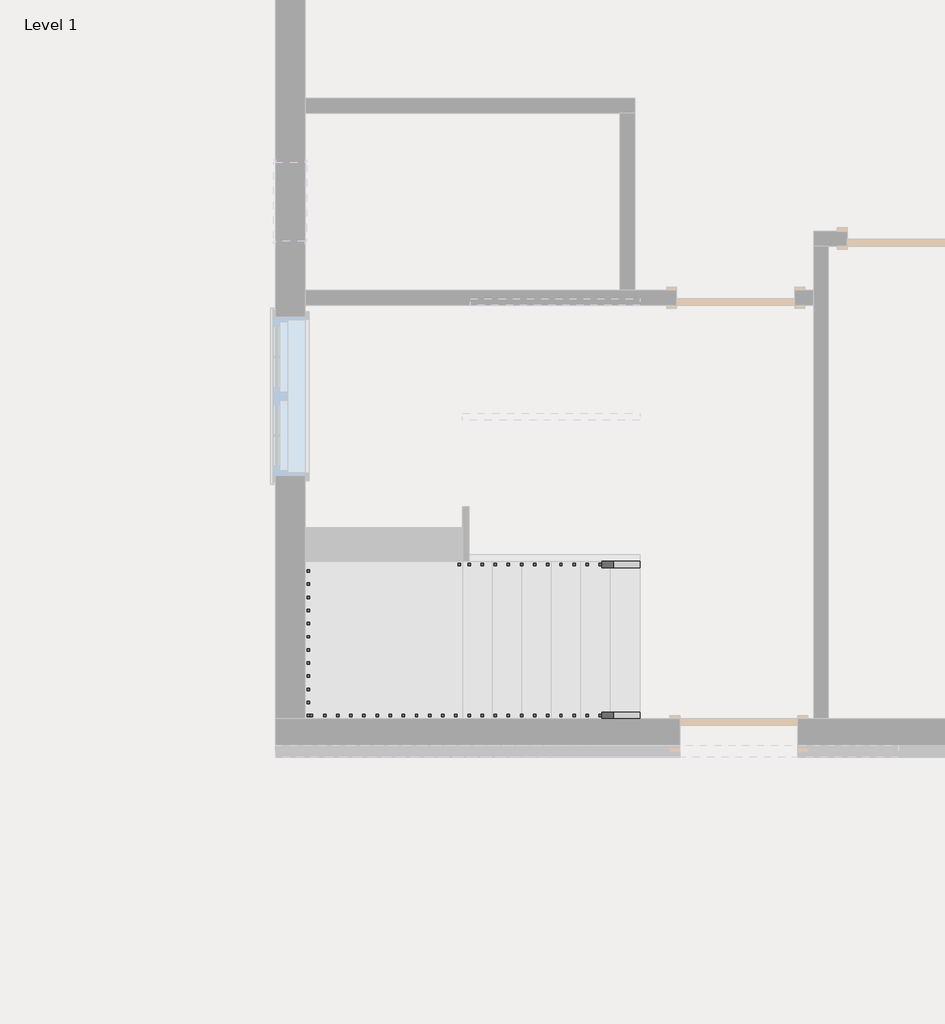
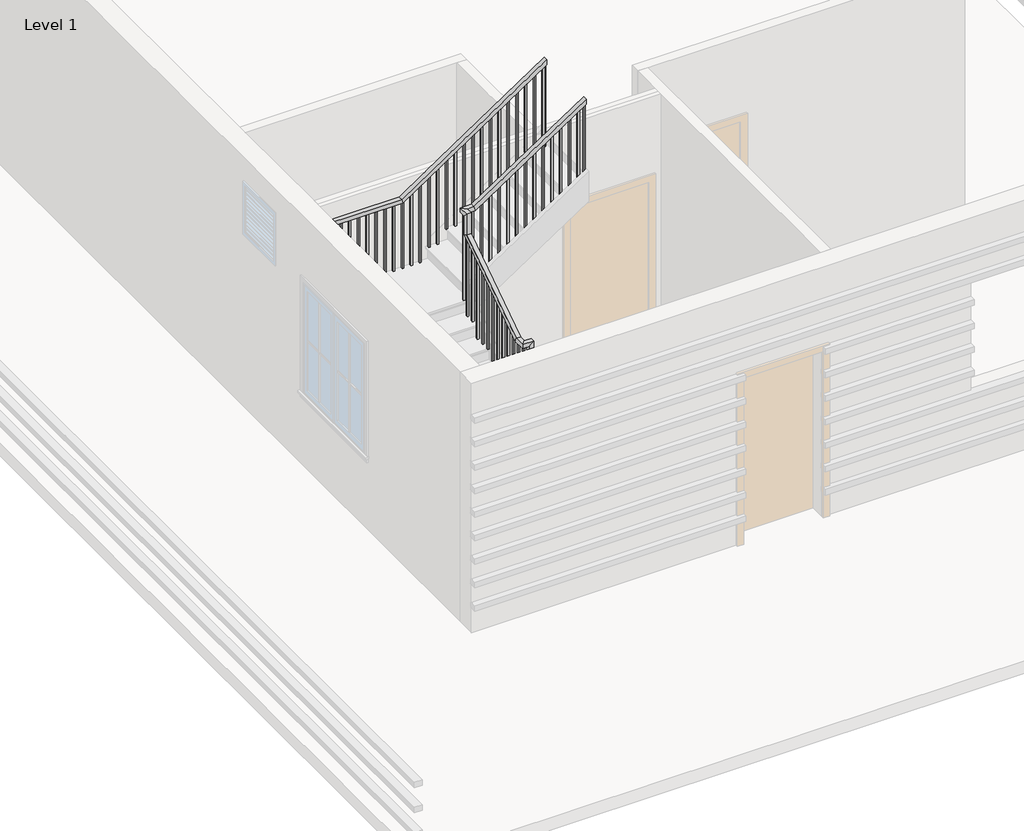
# One storey, part 3 of 4: 2 railings.
"""IFC4 building model written with IfcOpenShell, lengths in millimetres."""

from ifc_helpers import new_model, si_unit, frame, origin, place, context, project, spatial, polyline, outline, extrude, faceted_brep, element, save

model = new_model("IFC4")

# Units and contexts
model_context = context("Model", 3, world=origin())
ifc_project = project(units=[si_unit("LENGTHUNIT", "METRE", prefix="MILLI")], contexts=[model_context])

# Site, building, storey
site = spatial("IfcSite", under=ifc_project)
building = spatial("IfcBuilding", under=site)
storey = spatial("IfcBuildingStorey", under=building, Name="Level 1", Elevation=0.0)

# Railings
placement = place(None, origin())
element("IfcRailing", 1, ObjectType="Handrail - Rectangular", at=placement, inside=storey, context=model_context, shape_type="SolidModel", body=[
    faceted_brep([(-2515.2117403, -5213.8426559, 1066.8), (-2515.2117403, -5213.8426559, 1005.7459984), (-2515.2117403, -5163.0426559, 1005.7459984), (-2515.2117403, -5163.0426559, 1066.8), (-3810.6117403, -5213.8426559, 1930.4), (-3861.4117403, -5213.8426559, 1903.2126651), (-3861.4117403, -5163.0426559, 1903.2126651), (-3810.6117403, -5163.0426559, 1930.4), (-3810.6117403, -5213.8426559, 2184.4), (-3861.4117403, -5213.8426559, 2133.6), (-3861.4117403, -5163.0426559, 2133.6), (-3810.6117403, -5163.0426559, 2184.4), (-3937.6117403, -5213.8426559, 2184.4), (-3937.6117403, -5213.8426559, 2133.6), (-3886.8117403, -5163.0426559, 2133.6), (-3886.8117403, -5163.0426559, 2184.4), (-3937.6117403, -5086.8426559, 2184.4), (-3937.6117403, -5071.4616535, 2133.6), (-3886.8117403, -5071.4616535, 2133.6), (-3886.8117403, -5086.8426559, 2184.4), (-3937.6117403, -4096.2426559, 2844.8), (-3937.6117403, -4045.4426559, 2817.6126651), (-3886.8117403, -4045.4426559, 2817.6126651), (-3886.8117403, -4096.2426559, 2844.8), (-3937.6117403, -4096.2426559, 3098.8), (-3937.6117403, -4045.4426559, 3048.0), (-3886.8117403, -4045.4426559, 3048.0), (-3886.8117403, -4096.2426559, 3098.8), (-3937.6117403, -3969.2426559, 3098.8), (-3937.6117403, -3969.2426559, 3048.0), (-3886.8117403, -4020.0426559, 3048.0), (-3886.8117403, -4020.0426559, 3098.8), (-3810.6117403, -3969.2426559, 3098.8), (-3795.2307379, -3969.2426559, 3048.0), (-3795.2307379, -4020.0426559, 3048.0), (-3810.6117403, -4020.0426559, 3098.8), (-2515.2117403, -3969.2426559, 3962.4), (-2515.2117403, -4020.0426559, 3962.4), (-2515.2117403, -4020.0426559, 3901.3459984), (-2515.2117403, -3969.2426559, 3901.3459984)], [[[0, 1, 2, 3]], [[1, 0, 4, 5]], [[2, 1, 5, 6]], [[3, 2, 6, 7]], [[0, 3, 7, 4]], [[5, 4, 8, 9]], [[6, 5, 9, 10]], [[7, 6, 10, 11]], [[4, 7, 11, 8]], [[9, 8, 12, 13]], [[10, 9, 13, 14]], [[11, 10, 14, 15]], [[8, 11, 15, 12]], [[13, 12, 16, 17]], [[14, 13, 17, 18]], [[15, 14, 18, 19]], [[12, 15, 19, 16]], [[17, 16, 20, 21]], [[18, 17, 21, 22]], [[19, 18, 22, 23]], [[16, 19, 23, 20]], [[21, 20, 24, 25]], [[22, 21, 25, 26]], [[23, 22, 26, 27]], [[20, 23, 27, 24]], [[25, 24, 28, 29]], [[26, 25, 29, 30]], [[27, 26, 30, 31]], [[24, 27, 31, 28]], [[29, 28, 32, 33]], [[30, 29, 33, 34]], [[31, 30, 34, 35]], [[28, 31, 35, 32]], [[36, 37, 38, 39]], [[33, 32, 36, 39]], [[34, 33, 39, 38]], [[35, 34, 38, 37]], [[32, 35, 37, 36]]]),
    extrude(outline(polyline([(3856.8959984, -2581.8867403), (3844.1959984, -2600.9367403), (2895.6, -2600.9367403), (2895.6, -2581.8867403), (3856.8959984, -2581.8867403)])), frame((0.0, -4004.1676559, 0.0), z_axis=(0.0, 1.0, 0.0), x_axis=(0.0, 0.0, 1.0)), (0.0, 0.0, 1.0), 19.05),
    extrude(outline(polyline([(3789.1626651, -2683.4867403), (3776.4626651, -2702.5367403), (2895.6, -2702.5367403), (2895.6, -2683.4867403), (3789.1626651, -2683.4867403)])), frame((0.0, -4004.1676559, 0.0), z_axis=(0.0, 1.0, 0.0), x_axis=(0.0, 0.0, 1.0)), (0.0, 0.0, 1.0), 19.05),
    extrude(outline(polyline([(3721.4293317, -2785.0867403), (3708.7293317, -2804.1367403), (2743.2, -2804.1367403), (2743.2, -2785.0867403), (3721.4293317, -2785.0867403)])), frame((0.0, -4004.1676559, 0.0), z_axis=(0.0, 1.0, 0.0), x_axis=(0.0, 0.0, 1.0)), (0.0, 0.0, 1.0), 19.05),
    extrude(outline(polyline([(3653.6959984, -2886.6867403), (3640.9959984, -2905.7367403), (2743.2, -2905.7367403), (2743.2, -2886.6867403), (3653.6959984, -2886.6867403)])), frame((0.0, -4004.1676559, 0.0), z_axis=(0.0, 1.0, 0.0), x_axis=(0.0, 0.0, 1.0)), (0.0, 0.0, 1.0), 19.05),
    extrude(outline(polyline([(3585.9626651, -2988.2867403), (3573.2626651, -3007.3367403), (2590.8, -3007.3367403), (2590.8, -2988.2867403), (3585.9626651, -2988.2867403)])), frame((0.0, -4004.1676559, 0.0), z_axis=(0.0, 1.0, 0.0), x_axis=(0.0, 0.0, 1.0)), (0.0, 0.0, 1.0), 19.05),
    extrude(outline(polyline([(3518.2293317, -3089.8867403), (3505.5293317, -3108.9367403), (2590.8, -3108.9367403), (2590.8, -3089.8867403), (3518.2293317, -3089.8867403)])), frame((0.0, -4004.1676559, 0.0), z_axis=(0.0, 1.0, 0.0), x_axis=(0.0, 0.0, 1.0)), (0.0, 0.0, 1.0), 19.05),
    extrude(outline(polyline([(3450.4959984, -3191.4867403), (3437.7959984, -3210.5367403), (2590.8, -3210.5367403), (2590.8, -3191.4867403), (3450.4959984, -3191.4867403)])), frame((0.0, -4004.1676559, 0.0), z_axis=(0.0, 1.0, 0.0), x_axis=(0.0, 0.0, 1.0)), (0.0, 0.0, 1.0), 19.05),
    extrude(outline(polyline([(3382.7626651, -3293.0867403), (3370.0626651, -3312.1367403), (2438.4, -3312.1367403), (2438.4, -3293.0867403), (3382.7626651, -3293.0867403)])), frame((0.0, -4004.1676559, 0.0), z_axis=(0.0, 1.0, 0.0), x_axis=(0.0, 0.0, 1.0)), (0.0, 0.0, 1.0), 19.05),
    extrude(outline(polyline([(3315.0293317, -3394.6867403), (3302.3293317, -3413.7367403), (2438.4, -3413.7367403), (2438.4, -3394.6867403), (3315.0293317, -3394.6867403)])), frame((0.0, -4004.1676559, 0.0), z_axis=(0.0, 1.0, 0.0), x_axis=(0.0, 0.0, 1.0)), (0.0, 0.0, 1.0), 19.05),
    extrude(outline(polyline([(3247.2959984, -3496.2867403), (3234.5959984, -3515.3367403), (2286.0, -3515.3367403), (2286.0, -3496.2867403), (3247.2959984, -3496.2867403)])), frame((0.0, -4004.1676559, 0.0), z_axis=(0.0, 1.0, 0.0), x_axis=(0.0, 0.0, 1.0)), (0.0, 0.0, 1.0), 19.05),
    extrude(outline(polyline([(3179.5626651, -3597.8867403), (3166.8626651, -3616.9367403), (2286.0, -3616.9367403), (2286.0, -3597.8867403), (3179.5626651, -3597.8867403)])), frame((0.0, -4004.1676559, 0.0), z_axis=(0.0, 1.0, 0.0), x_axis=(0.0, 0.0, 1.0)), (0.0, 0.0, 1.0), 19.05),
    extrude(outline(polyline([(3111.8293317, -3699.4867403), (3099.1293317, -3718.5367403), (2133.6, -3718.5367403), (2133.6, -3699.4867403), (3111.8293317, -3699.4867403)])), frame((0.0, -4004.1676559, 0.0), z_axis=(0.0, 1.0, 0.0), x_axis=(0.0, 0.0, 1.0)), (0.0, 0.0, 1.0), 19.05),
    extrude(outline(polyline([(3044.0959984, -3801.0867403), (3031.3959984, -3820.1367403), (2133.6, -3820.1367403), (2133.6, -3801.0867403), (3044.0959984, -3801.0867403)])), frame((0.0, -4004.1676559, 0.0), z_axis=(0.0, 1.0, 0.0), x_axis=(0.0, 0.0, 1.0)), (0.0, 0.0, 1.0), 19.05),
    extrude(outline(polyline([(-3902.6867403, -4080.3676559), (-3921.7367403, -4080.3676559), (-3921.7367403, -4061.3176559), (-3902.6867403, -4061.3176559), (-3902.6867403, -4080.3676559)])), frame((0.0, 0.0, 1828.8), z_axis=(0.0, 0.0, 1.0), x_axis=(1.0, 0.0, 0.0)), (0.0, 0.0, 1.0), 1219.2),
    extrude(outline(polyline([(-4181.9676559, 2726.5959984), (-4162.9176559, 2739.2959984), (-4162.9176559, 1828.8), (-4181.9676559, 1828.8), (-4181.9676559, 2726.5959984)])), frame((-3921.7367403, 0.0, 0.0), z_axis=(1.0, 0.0, 0.0), x_axis=(0.0, 1.0, 0.0)), (0.0, 0.0, 1.0), 19.05),
    extrude(outline(polyline([(-4283.5676559, 2658.8626651), (-4264.5176559, 2671.5626651), (-4264.5176559, 1676.4), (-4283.5676559, 1676.4), (-4283.5676559, 2658.8626651)])), frame((-3921.7367403, 0.0, 0.0), z_axis=(1.0, 0.0, 0.0), x_axis=(0.0, 1.0, 0.0)), (0.0, 0.0, 1.0), 19.05),
    extrude(outline(polyline([(-4385.1676559, 2591.1293317), (-4366.1176559, 2603.8293317), (-4366.1176559, 1676.4), (-4385.1676559, 1676.4), (-4385.1676559, 2591.1293317)])), frame((-3921.7367403, 0.0, 0.0), z_axis=(1.0, 0.0, 0.0), x_axis=(0.0, 1.0, 0.0)), (0.0, 0.0, 1.0), 19.05),
    extrude(outline(polyline([(-4486.7676559, 2523.3959984), (-4467.7176559, 2536.0959984), (-4467.7176559, 1676.4), (-4486.7676559, 1676.4), (-4486.7676559, 2523.3959984)])), frame((-3921.7367403, 0.0, 0.0), z_axis=(1.0, 0.0, 0.0), x_axis=(0.0, 1.0, 0.0)), (0.0, 0.0, 1.0), 19.05),
    extrude(outline(polyline([(-4588.3676559, 2455.6626651), (-4569.3176559, 2468.3626651), (-4569.3176559, 1524.0), (-4588.3676559, 1524.0), (-4588.3676559, 2455.6626651)])), frame((-3921.7367403, 0.0, 0.0), z_axis=(1.0, 0.0, 0.0), x_axis=(0.0, 1.0, 0.0)), (0.0, 0.0, 1.0), 19.05),
    extrude(outline(polyline([(-4689.9676559, 2387.9293317), (-4670.9176559, 2400.6293317), (-4670.9176559, 1524.0), (-4689.9676559, 1524.0), (-4689.9676559, 2387.9293317)])), frame((-3921.7367403, 0.0, 0.0), z_axis=(1.0, 0.0, 0.0), x_axis=(0.0, 1.0, 0.0)), (0.0, 0.0, 1.0), 19.05),
    extrude(outline(polyline([(-4791.5676559, 2320.1959984), (-4772.5176559, 2332.8959984), (-4772.5176559, 1371.6), (-4791.5676559, 1371.6), (-4791.5676559, 2320.1959984)])), frame((-3921.7367403, 0.0, 0.0), z_axis=(1.0, 0.0, 0.0), x_axis=(0.0, 1.0, 0.0)), (0.0, 0.0, 1.0), 19.05),
    extrude(outline(polyline([(-4893.1676559, 2252.4626651), (-4874.1176559, 2265.1626651), (-4874.1176559, 1371.6), (-4893.1676559, 1371.6), (-4893.1676559, 2252.4626651)])), frame((-3921.7367403, 0.0, 0.0), z_axis=(1.0, 0.0, 0.0), x_axis=(0.0, 1.0, 0.0)), (0.0, 0.0, 1.0), 19.05),
    extrude(outline(polyline([(-4994.7676559, 2184.7293317), (-4975.7176559, 2197.4293317), (-4975.7176559, 1219.2), (-4994.7676559, 1219.2), (-4994.7676559, 2184.7293317)])), frame((-3921.7367403, 0.0, 0.0), z_axis=(1.0, 0.0, 0.0), x_axis=(0.0, 1.0, 0.0)), (0.0, 0.0, 1.0), 19.05),
    extrude(outline(polyline([(-5096.3676559, 2116.9959984), (-5077.3176559, 2129.6959984), (-5077.3176559, 1219.2), (-5096.3676559, 1219.2), (-5096.3676559, 2116.9959984)])), frame((-3921.7367403, 0.0, 0.0), z_axis=(1.0, 0.0, 0.0), x_axis=(0.0, 1.0, 0.0)), (0.0, 0.0, 1.0), 19.05),
    extrude(outline(polyline([(-3826.4867403, -5178.9176559), (-3826.4867403, -5197.9676559), (-3845.5367403, -5197.9676559), (-3845.5367403, -5178.9176559), (-3826.4867403, -5178.9176559)])), frame((0.0, 0.0, 914.4), z_axis=(0.0, 0.0, 1.0), x_axis=(1.0, 0.0, 0.0)), (0.0, 0.0, 1.0), 1219.2),
    extrude(outline(polyline([(1812.1959984, -3724.8867403), (1824.8959984, -3743.9367403), (914.4, -3743.9367403), (914.4, -3724.8867403), (1812.1959984, -3724.8867403)])), frame((0.0, -5197.9676559, 0.0), z_axis=(0.0, 1.0, 0.0), x_axis=(0.0, 0.0, 1.0)), (0.0, 0.0, 1.0), 19.05),
    extrude(outline(polyline([(1744.4626651, -3623.2867403), (1757.1626651, -3642.3367403), (762.0, -3642.3367403), (762.0, -3623.2867403), (1744.4626651, -3623.2867403)])), frame((0.0, -5197.9676559, 0.0), z_axis=(0.0, 1.0, 0.0), x_axis=(0.0, 0.0, 1.0)), (0.0, 0.0, 1.0), 19.05),
    extrude(outline(polyline([(1676.7293317, -3521.6867403), (1689.4293317, -3540.7367403), (762.0, -3540.7367403), (762.0, -3521.6867403), (1676.7293317, -3521.6867403)])), frame((0.0, -5197.9676559, 0.0), z_axis=(0.0, 1.0, 0.0), x_axis=(0.0, 0.0, 1.0)), (0.0, 0.0, 1.0), 19.05),
    extrude(outline(polyline([(1608.9959984, -3420.0867403), (1621.6959984, -3439.1367403), (762.0, -3439.1367403), (762.0, -3420.0867403), (1608.9959984, -3420.0867403)])), frame((0.0, -5197.9676559, 0.0), z_axis=(0.0, 1.0, 0.0), x_axis=(0.0, 0.0, 1.0)), (0.0, 0.0, 1.0), 19.05),
    extrude(outline(polyline([(1541.2626651, -3318.4867403), (1553.9626651, -3337.5367403), (609.6, -3337.5367403), (609.6, -3318.4867403), (1541.2626651, -3318.4867403)])), frame((0.0, -5197.9676559, 0.0), z_axis=(0.0, 1.0, 0.0), x_axis=(0.0, 0.0, 1.0)), (0.0, 0.0, 1.0), 19.05),
    extrude(outline(polyline([(1473.5293317, -3216.8867403), (1486.2293317, -3235.9367403), (609.6, -3235.9367403), (609.6, -3216.8867403), (1473.5293317, -3216.8867403)])), frame((0.0, -5197.9676559, 0.0), z_axis=(0.0, 1.0, 0.0), x_axis=(0.0, 0.0, 1.0)), (0.0, 0.0, 1.0), 19.05),
    extrude(outline(polyline([(1405.7959984, -3115.2867403), (1418.4959984, -3134.3367403), (457.2, -3134.3367403), (457.2, -3115.2867403), (1405.7959984, -3115.2867403)])), frame((0.0, -5197.9676559, 0.0), z_axis=(0.0, 1.0, 0.0), x_axis=(0.0, 0.0, 1.0)), (0.0, 0.0, 1.0), 19.05),
    extrude(outline(polyline([(1338.0626651, -3013.6867403), (1350.7626651, -3032.7367403), (457.2, -3032.7367403), (457.2, -3013.6867403), (1338.0626651, -3013.6867403)])), frame((0.0, -5197.9676559, 0.0), z_axis=(0.0, 1.0, 0.0), x_axis=(0.0, 0.0, 1.0)), (0.0, 0.0, 1.0), 19.05),
    extrude(outline(polyline([(1270.3293317, -2912.0867403), (1283.0293317, -2931.1367403), (304.8, -2931.1367403), (304.8, -2912.0867403), (1270.3293317, -2912.0867403)])), frame((0.0, -5197.9676559, 0.0), z_axis=(0.0, 1.0, 0.0), x_axis=(0.0, 0.0, 1.0)), (0.0, 0.0, 1.0), 19.05),
    extrude(outline(polyline([(1202.5959984, -2810.4867403), (1215.2959984, -2829.5367403), (304.8, -2829.5367403), (304.8, -2810.4867403), (1202.5959984, -2810.4867403)])), frame((0.0, -5197.9676559, 0.0), z_axis=(0.0, 1.0, 0.0), x_axis=(0.0, 0.0, 1.0)), (0.0, 0.0, 1.0), 19.05),
    extrude(outline(polyline([(1134.8626651, -2708.8867403), (1147.5626651, -2727.9367403), (152.4, -2727.9367403), (152.4, -2708.8867403), (1134.8626651, -2708.8867403)])), frame((0.0, -5197.9676559, 0.0), z_axis=(0.0, 1.0, 0.0), x_axis=(0.0, 0.0, 1.0)), (0.0, 0.0, 1.0), 19.05),
    extrude(outline(polyline([(1067.1293317, -2607.2867403), (1079.8293317, -2626.3367403), (152.4, -2626.3367403), (152.4, -2607.2867403), (1067.1293317, -2607.2867403)])), frame((0.0, -5197.9676559, 0.0), z_axis=(0.0, 1.0, 0.0), x_axis=(0.0, 0.0, 1.0)), (0.0, 0.0, 1.0), 19.05),
    extrude(outline(polyline([(-3902.6867403, -4004.1676559), (-3921.7367403, -4004.1676559), (-3921.7367403, -3985.1176559), (-3902.6867403, -3985.1176559), (-3902.6867403, -4004.1676559)])), frame((0.0, 0.0, 1981.2), z_axis=(0.0, 0.0, 1.0), x_axis=(1.0, 0.0, 0.0)), (0.0, 0.0, 1.0), 1066.8),
    extrude(outline(polyline([(-3902.6867403, -5178.9176559), (-3902.6867403, -5197.9676559), (-3921.7367403, -5197.9676559), (-3921.7367403, -5178.9176559), (-3902.6867403, -5178.9176559)])), frame((0.0, 0.0, 1066.8), z_axis=(0.0, 0.0, 1.0), x_axis=(1.0, 0.0, 0.0)), (0.0, 0.0, 1.0), 1066.8),
    extrude(outline(polyline([(3901.3459984, -2515.2117403), (3888.6459984, -2534.2617403), (2895.6, -2534.2617403), (2895.6, -2515.2117403), (3901.3459984, -2515.2117403)])), frame((0.0, -4004.1676559, 0.0), z_axis=(0.0, 1.0, 0.0), x_axis=(0.0, 0.0, 1.0)), (0.0, 0.0, 1.0), 19.05),
    extrude(outline(polyline([(1005.7459984, -2515.2117403), (1018.4459984, -2534.2617403), (152.4, -2534.2617403), (152.4, -2515.2117403), (1005.7459984, -2515.2117403)])), frame((0.0, -5197.9676559, 0.0), z_axis=(0.0, 1.0, 0.0), x_axis=(0.0, 0.0, 1.0)), (0.0, 0.0, 1.0), 19.05),
])
element("IfcRailing", 2, ObjectType="Handrail - Rectangular", at=placement, inside=storey, context=model_context, shape_type="SolidModel", body=[
    faceted_brep([(-2515.2117403, -6382.2426559, 1066.8), (-2515.2117403, -6382.2426559, 1005.7459984), (-2515.2117403, -6331.4426559, 1005.7459984), (-2515.2117403, -6331.4426559, 1066.8), (-4001.1117403, -6382.2426559, 2057.4), (-4016.4927427, -6382.2426559, 2006.6), (-4016.4927427, -6331.4426559, 2006.6), (-4001.1117403, -6331.4426559, 2057.4), (-5106.0117403, -6382.2426559, 2057.4), (-5106.0117403, -6382.2426559, 2006.6), (-5055.2117403, -6331.4426559, 2006.6), (-5055.2117403, -6331.4426559, 2057.4), (-5106.0117403, -5277.3426559, 2057.4), (-5106.0117403, -5261.9616535, 2006.6), (-5055.2117403, -5261.9616535, 2006.6), (-5055.2117403, -5277.3426559, 2057.4), (-5106.0117403, -4096.2426559, 2844.8), (-5106.0117403, -4080.8616535, 2794.0), (-5055.2117403, -4080.8616535, 2794.0), (-5055.2117403, -4096.2426559, 2844.8), (-5106.0117403, -3181.8426559, 2844.8), (-5106.0117403, -3181.8426559, 2794.0), (-5055.2117403, -3232.6426559, 2794.0), (-5055.2117403, -3232.6426559, 2844.8), (-4191.6117403, -3181.8426559, 2844.8), (-4176.2307379, -3181.8426559, 2794.0), (-4176.2307379, -3232.6426559, 2794.0), (-4191.6117403, -3232.6426559, 2844.8), (-2515.2117403, -3181.8426559, 3962.4), (-2515.2117403, -3232.6426559, 3962.4), (-2515.2117403, -3232.6426559, 3901.3459984), (-2515.2117403, -3181.8426559, 3901.3459984)], [[[0, 1, 2, 3]], [[1, 0, 4, 5]], [[2, 1, 5, 6]], [[3, 2, 6, 7]], [[0, 3, 7, 4]], [[5, 4, 8, 9]], [[6, 5, 9, 10]], [[7, 6, 10, 11]], [[4, 7, 11, 8]], [[9, 8, 12, 13]], [[10, 9, 13, 14]], [[11, 10, 14, 15]], [[8, 11, 15, 12]], [[13, 12, 16, 17]], [[14, 13, 17, 18]], [[15, 14, 18, 19]], [[12, 15, 19, 16]], [[17, 16, 20, 21]], [[18, 17, 21, 22]], [[19, 18, 22, 23]], [[16, 19, 23, 20]], [[21, 20, 24, 25]], [[22, 21, 25, 26]], [[23, 22, 26, 27]], [[20, 23, 27, 24]], [[28, 29, 30, 31]], [[25, 24, 28, 31]], [[26, 25, 31, 30]], [[27, 26, 30, 29]], [[24, 27, 29, 28]]]),
    extrude(outline(polyline([(3878.0626651, -2550.1367403), (2895.6, -2550.1367403), (2895.6, -2531.0867403), (3890.7626651, -2531.0867403), (3878.0626651, -2550.1367403)])), frame((0.0, -3216.7676559, 0.0), z_axis=(0.0, 1.0, 0.0), x_axis=(0.0, 0.0, 1.0)), (0.0, 0.0, 1.0), 19.05),
    extrude(outline(polyline([(3810.3293317, -2651.7367403), (2895.6, -2651.7367403), (2895.6, -2632.6867403), (3823.0293317, -2632.6867403), (3810.3293317, -2651.7367403)])), frame((0.0, -3216.7676559, 0.0), z_axis=(0.0, 1.0, 0.0), x_axis=(0.0, 0.0, 1.0)), (0.0, 0.0, 1.0), 19.05),
    extrude(outline(polyline([(3742.5959984, -2753.3367403), (2895.6, -2753.3367403), (2895.6, -2734.2867403), (3755.2959984, -2734.2867403), (3742.5959984, -2753.3367403)])), frame((0.0, -3216.7676559, 0.0), z_axis=(0.0, 1.0, 0.0), x_axis=(0.0, 0.0, 1.0)), (0.0, 0.0, 1.0), 19.05),
    extrude(outline(polyline([(3674.8626651, -2854.9367403), (2743.2, -2854.9367403), (2743.2, -2835.8867403), (3687.5626651, -2835.8867403), (3674.8626651, -2854.9367403)])), frame((0.0, -3216.7676559, 0.0), z_axis=(0.0, 1.0, 0.0), x_axis=(0.0, 0.0, 1.0)), (0.0, 0.0, 1.0), 19.05),
    extrude(outline(polyline([(3607.1293317, -2956.5367403), (2743.2, -2956.5367403), (2743.2, -2937.4867403), (3619.8293317, -2937.4867403), (3607.1293317, -2956.5367403)])), frame((0.0, -3216.7676559, 0.0), z_axis=(0.0, 1.0, 0.0), x_axis=(0.0, 0.0, 1.0)), (0.0, 0.0, 1.0), 19.05),
    extrude(outline(polyline([(3539.3959984, -3058.1367403), (2590.8, -3058.1367403), (2590.8, -3039.0867403), (3552.0959984, -3039.0867403), (3539.3959984, -3058.1367403)])), frame((0.0, -3216.7676559, 0.0), z_axis=(0.0, 1.0, 0.0), x_axis=(0.0, 0.0, 1.0)), (0.0, 0.0, 1.0), 19.05),
    extrude(outline(polyline([(3471.6626651, -3159.7367403), (2590.8, -3159.7367403), (2590.8, -3140.6867403), (3484.3626651, -3140.6867403), (3471.6626651, -3159.7367403)])), frame((0.0, -3216.7676559, 0.0), z_axis=(0.0, 1.0, 0.0), x_axis=(0.0, 0.0, 1.0)), (0.0, 0.0, 1.0), 19.05),
    extrude(outline(polyline([(3403.9293317, -3261.3367403), (2438.4, -3261.3367403), (2438.4, -3242.2867403), (3416.6293317, -3242.2867403), (3403.9293317, -3261.3367403)])), frame((0.0, -3216.7676559, 0.0), z_axis=(0.0, 1.0, 0.0), x_axis=(0.0, 0.0, 1.0)), (0.0, 0.0, 1.0), 19.05),
    extrude(outline(polyline([(3336.1959984, -3362.9367403), (2438.4, -3362.9367403), (2438.4, -3343.8867403), (3348.8959984, -3343.8867403), (3336.1959984, -3362.9367403)])), frame((0.0, -3216.7676559, 0.0), z_axis=(0.0, 1.0, 0.0), x_axis=(0.0, 0.0, 1.0)), (0.0, 0.0, 1.0), 19.05),
    extrude(outline(polyline([(3268.4626651, -3464.5367403), (2286.0, -3464.5367403), (2286.0, -3445.4867403), (3281.1626651, -3445.4867403), (3268.4626651, -3464.5367403)])), frame((0.0, -3216.7676559, 0.0), z_axis=(0.0, 1.0, 0.0), x_axis=(0.0, 0.0, 1.0)), (0.0, 0.0, 1.0), 19.05),
    extrude(outline(polyline([(3200.7293317, -3566.1367403), (2286.0, -3566.1367403), (2286.0, -3547.0867403), (3213.4293317, -3547.0867403), (3200.7293317, -3566.1367403)])), frame((0.0, -3216.7676559, 0.0), z_axis=(0.0, 1.0, 0.0), x_axis=(0.0, 0.0, 1.0)), (0.0, 0.0, 1.0), 19.05),
    extrude(outline(polyline([(3132.9959984, -3667.7367403), (2286.0, -3667.7367403), (2286.0, -3648.6867403), (3145.6959984, -3648.6867403), (3132.9959984, -3667.7367403)])), frame((0.0, -3216.7676559, 0.0), z_axis=(0.0, 1.0, 0.0), x_axis=(0.0, 0.0, 1.0)), (0.0, 0.0, 1.0), 19.05),
    extrude(outline(polyline([(3065.2626651, -3769.3367403), (2133.6, -3769.3367403), (2133.6, -3750.2867403), (3077.9626651, -3750.2867403), (3065.2626651, -3769.3367403)])), frame((0.0, -3216.7676559, 0.0), z_axis=(0.0, 1.0, 0.0), x_axis=(0.0, 0.0, 1.0)), (0.0, 0.0, 1.0), 19.05),
    extrude(outline(polyline([(2997.5293317, -3870.9367403), (2133.6, -3870.9367403), (2133.6, -3851.8867403), (3010.2293317, -3851.8867403), (2997.5293317, -3870.9367403)])), frame((0.0, -3216.7676559, 0.0), z_axis=(0.0, 1.0, 0.0), x_axis=(0.0, 0.0, 1.0)), (0.0, 0.0, 1.0), 19.05),
    extrude(outline(polyline([(2929.7959984, -3972.5367403), (1981.2, -3972.5367403), (1981.2, -3953.4867403), (2942.4959984, -3953.4867403), (2929.7959984, -3972.5367403)])), frame((0.0, -3216.7676559, 0.0), z_axis=(0.0, 1.0, 0.0), x_axis=(0.0, 0.0, 1.0)), (0.0, 0.0, 1.0), 19.05),
    extrude(outline(polyline([(2862.0626651, -4074.1367403), (1981.2, -4074.1367403), (1981.2, -4055.0867403), (2874.7626651, -4055.0867403), (2862.0626651, -4074.1367403)])), frame((0.0, -3216.7676559, 0.0), z_axis=(0.0, 1.0, 0.0), x_axis=(0.0, 0.0, 1.0)), (0.0, 0.0, 1.0), 19.05),
    extrude(outline(polyline([(2794.3293317, -4175.7367403), (1981.2, -4175.7367403), (1981.2, -4156.6867403), (2807.0293317, -4156.6867403), (2794.3293317, -4175.7367403)])), frame((0.0, -3216.7676559, 0.0), z_axis=(0.0, 1.0, 0.0), x_axis=(0.0, 0.0, 1.0)), (0.0, 0.0, 1.0), 19.05),
    extrude(outline(polyline([(-4277.3367403, -3197.7176559), (-4258.2867403, -3197.7176559), (-4258.2867403, -3216.7676559), (-4277.3367403, -3216.7676559), (-4277.3367403, -3197.7176559)])), frame((0.0, 0.0, 1981.2), z_axis=(0.0, 0.0, 1.0), x_axis=(1.0, 0.0, 0.0)), (0.0, 0.0, 1.0), 812.8),
    extrude(outline(polyline([(-4378.9367403, -3197.7176559), (-4359.8867403, -3197.7176559), (-4359.8867403, -3216.7676559), (-4378.9367403, -3216.7676559), (-4378.9367403, -3197.7176559)])), frame((0.0, 0.0, 1981.2), z_axis=(0.0, 0.0, 1.0), x_axis=(1.0, 0.0, 0.0)), (0.0, 0.0, 1.0), 812.8),
    extrude(outline(polyline([(-4480.5367403, -3197.7176559), (-4461.4867403, -3197.7176559), (-4461.4867403, -3216.7676559), (-4480.5367403, -3216.7676559), (-4480.5367403, -3197.7176559)])), frame((0.0, 0.0, 1981.2), z_axis=(0.0, 0.0, 1.0), x_axis=(1.0, 0.0, 0.0)), (0.0, 0.0, 1.0), 812.8),
    extrude(outline(polyline([(-4582.1367403, -3197.7176559), (-4563.0867403, -3197.7176559), (-4563.0867403, -3216.7676559), (-4582.1367403, -3216.7676559), (-4582.1367403, -3197.7176559)])), frame((0.0, 0.0, 1981.2), z_axis=(0.0, 0.0, 1.0), x_axis=(1.0, 0.0, 0.0)), (0.0, 0.0, 1.0), 812.8),
    extrude(outline(polyline([(-4683.7367403, -3197.7176559), (-4664.6867403, -3197.7176559), (-4664.6867403, -3216.7676559), (-4683.7367403, -3216.7676559), (-4683.7367403, -3197.7176559)])), frame((0.0, 0.0, 1981.2), z_axis=(0.0, 0.0, 1.0), x_axis=(1.0, 0.0, 0.0)), (0.0, 0.0, 1.0), 812.8),
    extrude(outline(polyline([(-4785.3367403, -3197.7176559), (-4766.2867403, -3197.7176559), (-4766.2867403, -3216.7676559), (-4785.3367403, -3216.7676559), (-4785.3367403, -3197.7176559)])), frame((0.0, 0.0, 1981.2), z_axis=(0.0, 0.0, 1.0), x_axis=(1.0, 0.0, 0.0)), (0.0, 0.0, 1.0), 812.8),
    extrude(outline(polyline([(-4886.9367403, -3197.7176559), (-4867.8867403, -3197.7176559), (-4867.8867403, -3216.7676559), (-4886.9367403, -3216.7676559), (-4886.9367403, -3197.7176559)])), frame((0.0, 0.0, 1981.2), z_axis=(0.0, 0.0, 1.0), x_axis=(1.0, 0.0, 0.0)), (0.0, 0.0, 1.0), 812.8),
    extrude(outline(polyline([(-4988.5367403, -3197.7176559), (-4969.4867403, -3197.7176559), (-4969.4867403, -3216.7676559), (-4988.5367403, -3216.7676559), (-4988.5367403, -3197.7176559)])), frame((0.0, 0.0, 1981.2), z_axis=(0.0, 0.0, 1.0), x_axis=(1.0, 0.0, 0.0)), (0.0, 0.0, 1.0), 812.8),
    extrude(outline(polyline([(-5090.1367403, -3318.3676559), (-5090.1367403, -3299.3176559), (-5071.0867403, -3299.3176559), (-5071.0867403, -3318.3676559), (-5090.1367403, -3318.3676559)])), frame((0.0, 0.0, 1981.2), z_axis=(0.0, 0.0, 1.0), x_axis=(1.0, 0.0, 0.0)), (0.0, 0.0, 1.0), 812.8),
    extrude(outline(polyline([(-5090.1367403, -3419.9676559), (-5090.1367403, -3400.9176559), (-5071.0867403, -3400.9176559), (-5071.0867403, -3419.9676559), (-5090.1367403, -3419.9676559)])), frame((0.0, 0.0, 1981.2), z_axis=(0.0, 0.0, 1.0), x_axis=(1.0, 0.0, 0.0)), (0.0, 0.0, 1.0), 812.8),
    extrude(outline(polyline([(-5090.1367403, -3521.5676559), (-5090.1367403, -3502.5176559), (-5071.0867403, -3502.5176559), (-5071.0867403, -3521.5676559), (-5090.1367403, -3521.5676559)])), frame((0.0, 0.0, 1981.2), z_axis=(0.0, 0.0, 1.0), x_axis=(1.0, 0.0, 0.0)), (0.0, 0.0, 1.0), 812.8),
    extrude(outline(polyline([(-5090.1367403, -3623.1676559), (-5090.1367403, -3604.1176559), (-5071.0867403, -3604.1176559), (-5071.0867403, -3623.1676559), (-5090.1367403, -3623.1676559)])), frame((0.0, 0.0, 1981.2), z_axis=(0.0, 0.0, 1.0), x_axis=(1.0, 0.0, 0.0)), (0.0, 0.0, 1.0), 812.8),
    extrude(outline(polyline([(-5090.1367403, -3724.7676559), (-5090.1367403, -3705.7176559), (-5071.0867403, -3705.7176559), (-5071.0867403, -3724.7676559), (-5090.1367403, -3724.7676559)])), frame((0.0, 0.0, 1981.2), z_axis=(0.0, 0.0, 1.0), x_axis=(1.0, 0.0, 0.0)), (0.0, 0.0, 1.0), 812.8),
    extrude(outline(polyline([(-5090.1367403, -3826.3676559), (-5090.1367403, -3807.3176559), (-5071.0867403, -3807.3176559), (-5071.0867403, -3826.3676559), (-5090.1367403, -3826.3676559)])), frame((0.0, 0.0, 1981.2), z_axis=(0.0, 0.0, 1.0), x_axis=(1.0, 0.0, 0.0)), (0.0, 0.0, 1.0), 812.8),
    extrude(outline(polyline([(-5090.1367403, -3927.9676559), (-5090.1367403, -3908.9176559), (-5071.0867403, -3908.9176559), (-5071.0867403, -3927.9676559), (-5090.1367403, -3927.9676559)])), frame((0.0, 0.0, 1981.2), z_axis=(0.0, 0.0, 1.0), x_axis=(1.0, 0.0, 0.0)), (0.0, 0.0, 1.0), 812.8),
    extrude(outline(polyline([(-5090.1367403, -4029.5676559), (-5090.1367403, -4010.5176559), (-5071.0867403, -4010.5176559), (-5071.0867403, -4029.5676559), (-5090.1367403, -4029.5676559)])), frame((0.0, 0.0, 1981.2), z_axis=(0.0, 0.0, 1.0), x_axis=(1.0, 0.0, 0.0)), (0.0, 0.0, 1.0), 812.8),
    extrude(outline(polyline([(-4112.1176559, 2773.1626651), (-4112.1176559, 1828.8), (-4131.1676559, 1828.8), (-4131.1676559, 2760.4626651), (-4112.1176559, 2773.1626651)])), frame((-5090.1367403, 0.0, 0.0), z_axis=(1.0, 0.0, 0.0), x_axis=(0.0, 1.0, 0.0)), (0.0, 0.0, 1.0), 19.05),
    extrude(outline(polyline([(-4213.7176559, 2705.4293317), (-4213.7176559, 1828.8), (-4232.7676559, 1828.8), (-4232.7676559, 2692.7293317), (-4213.7176559, 2705.4293317)])), frame((-5090.1367403, 0.0, 0.0), z_axis=(1.0, 0.0, 0.0), x_axis=(0.0, 1.0, 0.0)), (0.0, 0.0, 1.0), 19.05),
    extrude(outline(polyline([(-4315.3176559, 2637.6959984), (-4315.3176559, 1676.4), (-4334.3676559, 1676.4), (-4334.3676559, 2624.9959984), (-4315.3176559, 2637.6959984)])), frame((-5090.1367403, 0.0, 0.0), z_axis=(1.0, 0.0, 0.0), x_axis=(0.0, 1.0, 0.0)), (0.0, 0.0, 1.0), 19.05),
    extrude(outline(polyline([(-4416.9176559, 2569.9626651), (-4416.9176559, 1676.4), (-4435.9676559, 1676.4), (-4435.9676559, 2557.2626651), (-4416.9176559, 2569.9626651)])), frame((-5090.1367403, 0.0, 0.0), z_axis=(1.0, 0.0, 0.0), x_axis=(0.0, 1.0, 0.0)), (0.0, 0.0, 1.0), 19.05),
    extrude(outline(polyline([(-4518.5176559, 2502.2293317), (-4518.5176559, 1524.0), (-4537.5676559, 1524.0), (-4537.5676559, 2489.5293317), (-4518.5176559, 2502.2293317)])), frame((-5090.1367403, 0.0, 0.0), z_axis=(1.0, 0.0, 0.0), x_axis=(0.0, 1.0, 0.0)), (0.0, 0.0, 1.0), 19.05),
    extrude(outline(polyline([(-4620.1176559, 2434.4959984), (-4620.1176559, 1524.0), (-4639.1676559, 1524.0), (-4639.1676559, 2421.7959984), (-4620.1176559, 2434.4959984)])), frame((-5090.1367403, 0.0, 0.0), z_axis=(1.0, 0.0, 0.0), x_axis=(0.0, 1.0, 0.0)), (0.0, 0.0, 1.0), 19.05),
    extrude(outline(polyline([(-4721.7176559, 2366.7626651), (-4721.7176559, 1371.6), (-4740.7676559, 1371.6), (-4740.7676559, 2354.0626651), (-4721.7176559, 2366.7626651)])), frame((-5090.1367403, 0.0, 0.0), z_axis=(1.0, 0.0, 0.0), x_axis=(0.0, 1.0, 0.0)), (0.0, 0.0, 1.0), 19.05),
    extrude(outline(polyline([(-4823.3176559, 2299.0293317), (-4823.3176559, 1371.6), (-4842.3676559, 1371.6), (-4842.3676559, 2286.3293317), (-4823.3176559, 2299.0293317)])), frame((-5090.1367403, 0.0, 0.0), z_axis=(1.0, 0.0, 0.0), x_axis=(0.0, 1.0, 0.0)), (0.0, 0.0, 1.0), 19.05),
    extrude(outline(polyline([(-4924.9176559, 2231.2959984), (-4924.9176559, 1371.6), (-4943.9676559, 1371.6), (-4943.9676559, 2218.5959984), (-4924.9176559, 2231.2959984)])), frame((-5090.1367403, 0.0, 0.0), z_axis=(1.0, 0.0, 0.0), x_axis=(0.0, 1.0, 0.0)), (0.0, 0.0, 1.0), 19.05),
    extrude(outline(polyline([(-5026.5176559, 2163.5626651), (-5026.5176559, 1219.2), (-5045.5676559, 1219.2), (-5045.5676559, 2150.8626651), (-5026.5176559, 2163.5626651)])), frame((-5090.1367403, 0.0, 0.0), z_axis=(1.0, 0.0, 0.0), x_axis=(0.0, 1.0, 0.0)), (0.0, 0.0, 1.0), 19.05),
    extrude(outline(polyline([(-5128.1176559, 2095.8293317), (-5128.1176559, 1219.2), (-5147.1676559, 1219.2), (-5147.1676559, 2083.1293317), (-5128.1176559, 2095.8293317)])), frame((-5090.1367403, 0.0, 0.0), z_axis=(1.0, 0.0, 0.0), x_axis=(0.0, 1.0, 0.0)), (0.0, 0.0, 1.0), 19.05),
    extrude(outline(polyline([(-5229.7176559, 2028.0959984), (-5229.7176559, 1066.8), (-5248.7676559, 1066.8), (-5248.7676559, 2015.3959984), (-5229.7176559, 2028.0959984)])), frame((-5090.1367403, 0.0, 0.0), z_axis=(1.0, 0.0, 0.0), x_axis=(0.0, 1.0, 0.0)), (0.0, 0.0, 1.0), 19.05),
    extrude(outline(polyline([(-5090.1367403, -5350.3676559), (-5090.1367403, -5331.3176559), (-5071.0867403, -5331.3176559), (-5071.0867403, -5350.3676559), (-5090.1367403, -5350.3676559)])), frame((0.0, 0.0, 1066.8), z_axis=(0.0, 0.0, 1.0), x_axis=(1.0, 0.0, 0.0)), (0.0, 0.0, 1.0), 939.8),
    extrude(outline(polyline([(-5090.1367403, -5451.9676559), (-5090.1367403, -5432.9176559), (-5071.0867403, -5432.9176559), (-5071.0867403, -5451.9676559), (-5090.1367403, -5451.9676559)])), frame((0.0, 0.0, 1066.8), z_axis=(0.0, 0.0, 1.0), x_axis=(1.0, 0.0, 0.0)), (0.0, 0.0, 1.0), 939.8),
    extrude(outline(polyline([(-5090.1367403, -5553.5676559), (-5090.1367403, -5534.5176559), (-5071.0867403, -5534.5176559), (-5071.0867403, -5553.5676559), (-5090.1367403, -5553.5676559)])), frame((0.0, 0.0, 1066.8), z_axis=(0.0, 0.0, 1.0), x_axis=(1.0, 0.0, 0.0)), (0.0, 0.0, 1.0), 939.8),
    extrude(outline(polyline([(-5090.1367403, -5655.1676559), (-5090.1367403, -5636.1176559), (-5071.0867403, -5636.1176559), (-5071.0867403, -5655.1676559), (-5090.1367403, -5655.1676559)])), frame((0.0, 0.0, 1066.8), z_axis=(0.0, 0.0, 1.0), x_axis=(1.0, 0.0, 0.0)), (0.0, 0.0, 1.0), 939.8),
    extrude(outline(polyline([(-5090.1367403, -5756.7676559), (-5090.1367403, -5737.7176559), (-5071.0867403, -5737.7176559), (-5071.0867403, -5756.7676559), (-5090.1367403, -5756.7676559)])), frame((0.0, 0.0, 1066.8), z_axis=(0.0, 0.0, 1.0), x_axis=(1.0, 0.0, 0.0)), (0.0, 0.0, 1.0), 939.8),
    extrude(outline(polyline([(-5090.1367403, -5858.3676559), (-5090.1367403, -5839.3176559), (-5071.0867403, -5839.3176559), (-5071.0867403, -5858.3676559), (-5090.1367403, -5858.3676559)])), frame((0.0, 0.0, 1066.8), z_axis=(0.0, 0.0, 1.0), x_axis=(1.0, 0.0, 0.0)), (0.0, 0.0, 1.0), 939.8),
    extrude(outline(polyline([(-5090.1367403, -5959.9676559), (-5090.1367403, -5940.9176559), (-5071.0867403, -5940.9176559), (-5071.0867403, -5959.9676559), (-5090.1367403, -5959.9676559)])), frame((0.0, 0.0, 1066.8), z_axis=(0.0, 0.0, 1.0), x_axis=(1.0, 0.0, 0.0)), (0.0, 0.0, 1.0), 939.8),
    extrude(outline(polyline([(-5090.1367403, -6061.5676559), (-5090.1367403, -6042.5176559), (-5071.0867403, -6042.5176559), (-5071.0867403, -6061.5676559), (-5090.1367403, -6061.5676559)])), frame((0.0, 0.0, 1066.8), z_axis=(0.0, 0.0, 1.0), x_axis=(1.0, 0.0, 0.0)), (0.0, 0.0, 1.0), 939.8),
    extrude(outline(polyline([(-5090.1367403, -6163.1676559), (-5090.1367403, -6144.1176559), (-5071.0867403, -6144.1176559), (-5071.0867403, -6163.1676559), (-5090.1367403, -6163.1676559)])), frame((0.0, 0.0, 1066.8), z_axis=(0.0, 0.0, 1.0), x_axis=(1.0, 0.0, 0.0)), (0.0, 0.0, 1.0), 939.8),
    extrude(outline(polyline([(-5090.1367403, -6264.7676559), (-5090.1367403, -6245.7176559), (-5071.0867403, -6245.7176559), (-5071.0867403, -6264.7676559), (-5090.1367403, -6264.7676559)])), frame((0.0, 0.0, 1066.8), z_axis=(0.0, 0.0, 1.0), x_axis=(1.0, 0.0, 0.0)), (0.0, 0.0, 1.0), 939.8),
    extrude(outline(polyline([(-5045.6867403, -6366.3676559), (-5064.7367403, -6366.3676559), (-5064.7367403, -6347.3176559), (-5045.6867403, -6347.3176559), (-5045.6867403, -6366.3676559)])), frame((0.0, 0.0, 1066.8), z_axis=(0.0, 0.0, 1.0), x_axis=(1.0, 0.0, 0.0)), (0.0, 0.0, 1.0), 939.8),
    extrude(outline(polyline([(-4944.0867403, -6366.3676559), (-4963.1367403, -6366.3676559), (-4963.1367403, -6347.3176559), (-4944.0867403, -6347.3176559), (-4944.0867403, -6366.3676559)])), frame((0.0, 0.0, 1066.8), z_axis=(0.0, 0.0, 1.0), x_axis=(1.0, 0.0, 0.0)), (0.0, 0.0, 1.0), 939.8),
    extrude(outline(polyline([(-4842.4867403, -6366.3676559), (-4861.5367403, -6366.3676559), (-4861.5367403, -6347.3176559), (-4842.4867403, -6347.3176559), (-4842.4867403, -6366.3676559)])), frame((0.0, 0.0, 1066.8), z_axis=(0.0, 0.0, 1.0), x_axis=(1.0, 0.0, 0.0)), (0.0, 0.0, 1.0), 939.8),
    extrude(outline(polyline([(-4740.8867403, -6366.3676559), (-4759.9367403, -6366.3676559), (-4759.9367403, -6347.3176559), (-4740.8867403, -6347.3176559), (-4740.8867403, -6366.3676559)])), frame((0.0, 0.0, 1066.8), z_axis=(0.0, 0.0, 1.0), x_axis=(1.0, 0.0, 0.0)), (0.0, 0.0, 1.0), 939.8),
    extrude(outline(polyline([(-4639.2867403, -6366.3676559), (-4658.3367403, -6366.3676559), (-4658.3367403, -6347.3176559), (-4639.2867403, -6347.3176559), (-4639.2867403, -6366.3676559)])), frame((0.0, 0.0, 1066.8), z_axis=(0.0, 0.0, 1.0), x_axis=(1.0, 0.0, 0.0)), (0.0, 0.0, 1.0), 939.8),
    extrude(outline(polyline([(-4537.6867403, -6366.3676559), (-4556.7367403, -6366.3676559), (-4556.7367403, -6347.3176559), (-4537.6867403, -6347.3176559), (-4537.6867403, -6366.3676559)])), frame((0.0, 0.0, 1066.8), z_axis=(0.0, 0.0, 1.0), x_axis=(1.0, 0.0, 0.0)), (0.0, 0.0, 1.0), 939.8),
    extrude(outline(polyline([(-4436.0867403, -6366.3676559), (-4455.1367403, -6366.3676559), (-4455.1367403, -6347.3176559), (-4436.0867403, -6347.3176559), (-4436.0867403, -6366.3676559)])), frame((0.0, 0.0, 1066.8), z_axis=(0.0, 0.0, 1.0), x_axis=(1.0, 0.0, 0.0)), (0.0, 0.0, 1.0), 939.8),
    extrude(outline(polyline([(-4334.4867403, -6366.3676559), (-4353.5367403, -6366.3676559), (-4353.5367403, -6347.3176559), (-4334.4867403, -6347.3176559), (-4334.4867403, -6366.3676559)])), frame((0.0, 0.0, 1066.8), z_axis=(0.0, 0.0, 1.0), x_axis=(1.0, 0.0, 0.0)), (0.0, 0.0, 1.0), 939.8),
    extrude(outline(polyline([(-4232.8867403, -6366.3676559), (-4251.9367403, -6366.3676559), (-4251.9367403, -6347.3176559), (-4232.8867403, -6347.3176559), (-4232.8867403, -6366.3676559)])), frame((0.0, 0.0, 1066.8), z_axis=(0.0, 0.0, 1.0), x_axis=(1.0, 0.0, 0.0)), (0.0, 0.0, 1.0), 939.8),
    extrude(outline(polyline([(-4131.2867403, -6366.3676559), (-4150.3367403, -6366.3676559), (-4150.3367403, -6347.3176559), (-4131.2867403, -6347.3176559), (-4131.2867403, -6366.3676559)])), frame((0.0, 0.0, 1066.8), z_axis=(0.0, 0.0, 1.0), x_axis=(1.0, 0.0, 0.0)), (0.0, 0.0, 1.0), 939.8),
    extrude(outline(polyline([(-4029.6867403, -6366.3676559), (-4048.7367403, -6366.3676559), (-4048.7367403, -6347.3176559), (-4029.6867403, -6347.3176559), (-4029.6867403, -6366.3676559)])), frame((0.0, 0.0, 1066.8), z_axis=(0.0, 0.0, 1.0), x_axis=(1.0, 0.0, 0.0)), (0.0, 0.0, 1.0), 939.8),
    extrude(outline(polyline([(1960.3626651, -3947.1367403), (1066.8, -3947.1367403), (1066.8, -3928.0867403), (1947.6626651, -3928.0867403), (1960.3626651, -3947.1367403)])), frame((0.0, -6366.3676559, 0.0), z_axis=(0.0, 1.0, 0.0), x_axis=(0.0, 0.0, 1.0)), (0.0, 0.0, 1.0), 19.05),
    extrude(outline(polyline([(1892.6293317, -3845.5367403), (914.4, -3845.5367403), (914.4, -3826.4867403), (1879.9293317, -3826.4867403), (1892.6293317, -3845.5367403)])), frame((0.0, -6366.3676559, 0.0), z_axis=(0.0, 1.0, 0.0), x_axis=(0.0, 0.0, 1.0)), (0.0, 0.0, 1.0), 19.05),
    extrude(outline(polyline([(1824.8959984, -3743.9367403), (914.4, -3743.9367403), (914.4, -3724.8867403), (1812.1959984, -3724.8867403), (1824.8959984, -3743.9367403)])), frame((0.0, -6366.3676559, 0.0), z_axis=(0.0, 1.0, 0.0), x_axis=(0.0, 0.0, 1.0)), (0.0, 0.0, 1.0), 19.05),
    extrude(outline(polyline([(1757.1626651, -3642.3367403), (762.0, -3642.3367403), (762.0, -3623.2867403), (1744.4626651, -3623.2867403), (1757.1626651, -3642.3367403)])), frame((0.0, -6366.3676559, 0.0), z_axis=(0.0, 1.0, 0.0), x_axis=(0.0, 0.0, 1.0)), (0.0, 0.0, 1.0), 19.05),
    extrude(outline(polyline([(1689.4293317, -3540.7367403), (762.0, -3540.7367403), (762.0, -3521.6867403), (1676.7293317, -3521.6867403), (1689.4293317, -3540.7367403)])), frame((0.0, -6366.3676559, 0.0), z_axis=(0.0, 1.0, 0.0), x_axis=(0.0, 0.0, 1.0)), (0.0, 0.0, 1.0), 19.05),
    extrude(outline(polyline([(1621.6959984, -3439.1367403), (762.0, -3439.1367403), (762.0, -3420.0867403), (1608.9959984, -3420.0867403), (1621.6959984, -3439.1367403)])), frame((0.0, -6366.3676559, 0.0), z_axis=(0.0, 1.0, 0.0), x_axis=(0.0, 0.0, 1.0)), (0.0, 0.0, 1.0), 19.05),
    extrude(outline(polyline([(1553.9626651, -3337.5367403), (609.6, -3337.5367403), (609.6, -3318.4867403), (1541.2626651, -3318.4867403), (1553.9626651, -3337.5367403)])), frame((0.0, -6366.3676559, 0.0), z_axis=(0.0, 1.0, 0.0), x_axis=(0.0, 0.0, 1.0)), (0.0, 0.0, 1.0), 19.05),
    extrude(outline(polyline([(1486.2293317, -3235.9367403), (609.6, -3235.9367403), (609.6, -3216.8867403), (1473.5293317, -3216.8867403), (1486.2293317, -3235.9367403)])), frame((0.0, -6366.3676559, 0.0), z_axis=(0.0, 1.0, 0.0), x_axis=(0.0, 0.0, 1.0)), (0.0, 0.0, 1.0), 19.05),
    extrude(outline(polyline([(1418.4959984, -3134.3367403), (457.2, -3134.3367403), (457.2, -3115.2867403), (1405.7959984, -3115.2867403), (1418.4959984, -3134.3367403)])), frame((0.0, -6366.3676559, 0.0), z_axis=(0.0, 1.0, 0.0), x_axis=(0.0, 0.0, 1.0)), (0.0, 0.0, 1.0), 19.05),
    extrude(outline(polyline([(1350.7626651, -3032.7367403), (457.2, -3032.7367403), (457.2, -3013.6867403), (1338.0626651, -3013.6867403), (1350.7626651, -3032.7367403)])), frame((0.0, -6366.3676559, 0.0), z_axis=(0.0, 1.0, 0.0), x_axis=(0.0, 0.0, 1.0)), (0.0, 0.0, 1.0), 19.05),
    extrude(outline(polyline([(1283.0293317, -2931.1367403), (304.8, -2931.1367403), (304.8, -2912.0867403), (1270.3293317, -2912.0867403), (1283.0293317, -2931.1367403)])), frame((0.0, -6366.3676559, 0.0), z_axis=(0.0, 1.0, 0.0), x_axis=(0.0, 0.0, 1.0)), (0.0, 0.0, 1.0), 19.05),
    extrude(outline(polyline([(1215.2959984, -2829.5367403), (304.8, -2829.5367403), (304.8, -2810.4867403), (1202.5959984, -2810.4867403), (1215.2959984, -2829.5367403)])), frame((0.0, -6366.3676559, 0.0), z_axis=(0.0, 1.0, 0.0), x_axis=(0.0, 0.0, 1.0)), (0.0, 0.0, 1.0), 19.05),
    extrude(outline(polyline([(1147.5626651, -2727.9367403), (152.4, -2727.9367403), (152.4, -2708.8867403), (1134.8626651, -2708.8867403), (1147.5626651, -2727.9367403)])), frame((0.0, -6366.3676559, 0.0), z_axis=(0.0, 1.0, 0.0), x_axis=(0.0, 0.0, 1.0)), (0.0, 0.0, 1.0), 19.05),
    extrude(outline(polyline([(1079.8293317, -2626.3367403), (152.4, -2626.3367403), (152.4, -2607.2867403), (1067.1293317, -2607.2867403), (1079.8293317, -2626.3367403)])), frame((0.0, -6366.3676559, 0.0), z_axis=(0.0, 1.0, 0.0), x_axis=(0.0, 0.0, 1.0)), (0.0, 0.0, 1.0), 19.05),
    extrude(outline(polyline([(-5090.1367403, -3216.7676559), (-5090.1367403, -3197.7176559), (-5071.0867403, -3197.7176559), (-5071.0867403, -3216.7676559), (-5090.1367403, -3216.7676559)])), frame((0.0, 0.0, 1981.2), z_axis=(0.0, 0.0, 1.0), x_axis=(1.0, 0.0, 0.0)), (0.0, 0.0, 1.0), 812.8),
    extrude(outline(polyline([(-5071.0867403, -6366.3676559), (-5090.1367403, -6366.3676559), (-5090.1367403, -6347.3176559), (-5071.0867403, -6347.3176559), (-5071.0867403, -6366.3676559)])), frame((0.0, 0.0, 1066.8), z_axis=(0.0, 0.0, 1.0), x_axis=(1.0, 0.0, 0.0)), (0.0, 0.0, 1.0), 939.8),
    extrude(outline(polyline([(3888.6459984, -2534.2617403), (2895.6, -2534.2617403), (2895.6, -2515.2117403), (3901.3459984, -2515.2117403), (3888.6459984, -2534.2617403)])), frame((0.0, -3216.7676559, 0.0), z_axis=(0.0, 1.0, 0.0), x_axis=(0.0, 0.0, 1.0)), (0.0, 0.0, 1.0), 19.05),
    extrude(outline(polyline([(1018.4459984, -2534.2617403), (152.4, -2534.2617403), (152.4, -2515.2117403), (1005.7459984, -2515.2117403), (1018.4459984, -2534.2617403)])), frame((0.0, -6366.3676559, 0.0), z_axis=(0.0, 1.0, 0.0), x_axis=(0.0, 0.0, 1.0)), (0.0, 0.0, 1.0), 19.05),
])

save(model, "model.ifc")

# Revit data of these elements
# Type "Handrail - Rectangular"
#   Assembly Code = "C2010400"
#   built-in parameter 1008612 = 0.0416667 (stored number, unit not read)
#   built-in parameter 1008611 = 0.0416667 (stored number, unit not read)
#   built-in parameter 1008609 = 0.333333 (stored number, unit not read)
#   built-in parameter 1008604 = 0.166667 (stored number, unit not read)
#   built-in parameter 1008603 = 0.166667 (stored number, unit not read)
#   Railing Height = 3' - 0"
#   built-in parameter 1008630 = 2
#   built-in parameter 1008610 = 2
#   built-in parameter 1008618 = Baluster - Square : 3/4"
# Elements 1, 2 (IfcRailing, "Handrail - Rectangular")
#   Phase Created = New Construction
#   Materials on its faces: "Clad - White"
# Materials
#   "Clad - White": class "Wood", colour RGB 242 242 238, transparency 0, Cost = 0
